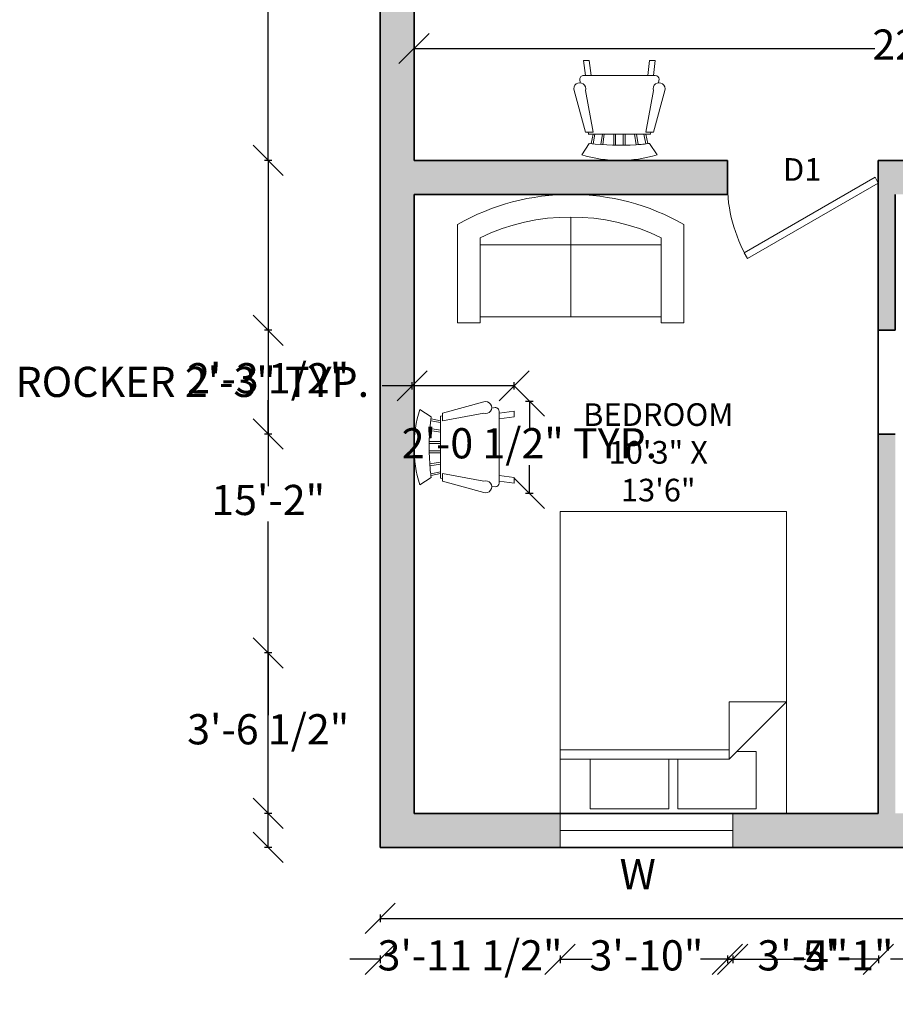
# Model space of a CAD drawing. Units: inches. Extents: x 2530 to 3100, y 543 to 1175.
# Tile 1 of 5: x 2530 to 2762, y 543 to 804. Entities that reach past the tile are written whole.
import ezdxf

# ---------------------------------------------------------------- set-up
doc = ezdxf.new("R2010")
doc.units = ezdxf.units.IN
for name, color, linetype, lineweight in [('A-ANNO-DIMS', 2, 'Continuous', 18), ('A-ANNO-TEXT', 7, 'Continuous', 18), ('A-AREA-IDEN', 7, 'Continuous', 18), ('A-DOOR', 3, 'Continuous', 18), ('A-FURN', 8, 'Continuous', 18), ('A-GLAZ', 4, 'Continuous', 18), ('A-WALL', 7, 'Continuous', 35), ('A-WALL-PATT', 30, 'Continuous', 13)]:
    doc.layers.add(name, color=color, linetype=linetype, lineweight=lineweight)
doc.styles.get("Standard").update_dxf_attribs({"font": 'arial.ttf'})
doc.dimstyles.new('ISO-25', dxfattribs={"dimtxt": 8, "dimasz": 8, "dimexe": 1, "dimexo": 1, "dimtad": 0, "dimtih": 1, "dimtoh": 1, "dimlunit": 3, "dimtxsty": 'Standard', "dimblk": 'OBLIQUE', "dimcen": 2.5, "dimadec": 0, "dimazin": 0, "dimtfac": 1, "dimtmove": 0, "dimatfit": 3, "dimfxl": 1, "dimfxlon": 1, "dimarcsym": 0})

# ---------------------------------------------------------------- blocks, each defined once
blk = doc.blocks.new('*U3')
for p, q in [((0, 0), (0, -6)), ((40, 0), (40, -6))]:
    blk.add_line(p, q)
blk.add_lwpolyline([(0, 0), (34.64, 20), (35.52, 18.48), (0.87, -1.52)], close=True)
blk.add_arc((0, 0), 40, 0, 30)
blk = doc.blocks.new('_Oblique')
at = {"color": 0, "linetype": 'ByBlock', "lineweight": -2}
blk.add_line((-0.5, -0.5), (0.5, 0.5), dxfattribs=at)
blk = doc.blocks.new('*D11')
at = {"layer": 'A-ANNO-DIMS', "color": 0, "lineweight": -2, "transparency": 16777216}
for p, q in [((2625.92, 566.6), (2625.92, 564.6)), ((3054.92, 566.6), (3054.92, 564.6)), ((2625.92, 565.6), (2826.05, 565.6)), ((3054.92, 565.6), (2854.78, 565.6))]:
    blk.add_line(p, q, dxfattribs=at)
at = {"layer": 'Defpoints', "color": 0, "transparency": 16777216}
for p in [(2625.92, 584.41), (3054.92, 584.41), (2625.92, 565.6)]:
    blk.add_point(p, dxfattribs=at)
at = {"layer": 'A-ANNO-DIMS', "color": 0, "lineweight": -2, "transparency": 16777216, "xscale": 8, "yscale": 8, "zscale": 8, "rotation": 180}
blk.add_blockref('_Oblique', (2625.92, 565.6), dxfattribs=at)
at = {"layer": 'A-ANNO-DIMS', "color": 0, "lineweight": -2, "transparency": 16777216, "xscale": 8, "yscale": 8, "zscale": 8}
blk.add_blockref('_Oblique', (3054.92, 565.6), dxfattribs=at)
at = {"layer": 'A-ANNO-DIMS', "color": 0, "transparency": 16777216, "insert": (2840.42, 565.6), "char_height": 8, "attachment_point": 5}
blk.add_mtext('35\'-9"', dxfattribs=at)
blk = doc.blocks.new('Chair - Rocking')
for p, q in [((-8, -4.5), (-10, -1.5)), ((8, -4.5), (10, -1.5)), ((-7.5, -4.5), (-7, -7)), ((-6.5, -7), (-7.02225, -4.43)), ((-4.5, -7), (-4.96674, -4.19951)), ((-4, -7), (-4.40532, -4.16272)), ((-1.5, -4.05012), (-1.5, -7)), ((-1, -7), (-1, -4.05012)), ((1, -7), (1, -4.04655)), ((1.5, -4.05012), (1.5, -7)), ((4, -7), (4.40187, -4.18694)), ((4.5, -7), (4.96761, -4.19437)), ((6.5, -7), (7, -4.4057)), ((7.5, -4.5), (7, -7)), ((-9, -7.5), (-12, -18.49999)), ((-7, -7.5), (-9, -7.5)), ((-9, -18.49999), (-7, -7.5)), ((-8.23428, -6.99939), (-8.3093, -7.47958)), ((-8.23041, -7), (8.23915, -7)), ((7, -7.5), (9, -7.5)), ((9, -18.49999), (7, -7.5)), ((8.31071, -7.48854), (8.23449, -7.00073)), ((9, -7.5), (12, -18.49999)), ((-10.36644, -20.64523), (-10.5, -21.49999)), ((10.5, -21.49999), (10.3575, -20.58798)), ((-9, -22.49999), (-9.5, -26.49999)), ((0, -22.49999), (-9.5, -22.49999)), ((-8, -26.49999), (-7.5, -22.49999)), ((0, -22.49999), (9.5, -22.49999)), ((8, -26.49999), (7.5, -22.49999)), ((9, -22.49999), (9.5, -26.49999)), ((-9.5, -26.49999), (-8, -26.49999)), ((9.5, -26.49999), (8, -26.49999))]:
    blk.add_line(p, q)
for centre, radius, start, end in [((0, -34.08333), 34.08333, 72.93847, 107.0615), ((0, -68.25004), 64.25, 93.92211, 97.15267), ((0, -68.25004), 64.25, 82.84733, 93.92211), ((-10.5, -18.99999), 1.58114, 161.5651, 18.43495), ((10.5, -18.99999), 1.58114, 161.5651, 18.43495), ((-9.5, -21.49999), 1, 180, 270), ((9.5, -21.49999), 1, 270, 0)]:
    blk.add_arc(centre, radius, start, end)
blk = doc.blocks.new('Bed - Queen')
for p, q in [((0, -80.00003), (0, 0)), ((0, 0), (59.99999, 0)), ((59.99999, 0), (59.99999, -80.00003)), ((7.99999, -1.2), (28.79998, -1.2)), ((7.99999, -14.4), (7.99999, -1.2)), ((28.79998, -1.2), (28.79998, -14.4)), ((31.19999, -1.2), (51.99999, -1.2)), ((31.19999, -14.4), (31.19999, -1.2)), ((51.99999, -1.2), (51.99999, -16.4)), ((0, -14.4), (44.8, -14.4)), ((59.99999, -29.6), (44.8, -14.4)), ((44.8, -14.4), (44.8, -29.6)), ((44.8, -16.8), (0, -16.8)), ((51.99999, -16.4), (46.79936, -16.4)), ((44.8, -29.6), (59.99999, -29.6)), ((59.99999, -80.00003), (0, -80.00003))]:
    blk.add_line(p, q)
blk = doc.blocks.new('Sofa - Roundback Loveseat 5 ft.')
for p, q in [((0, -32.44198), (0, -5.99998)), ((-24, -33.99998), (-24, -11.46958)), ((24.00004, -33.99998), (24.00004, -11.46958)), ((-23.9998, -13.38178), (23.99986, -13.38178)), ((-24, -32.44198), (24.00004, -32.44198))]:
    blk.add_line(p, q)
for points in [[(-24, -33.99998), (-30, -33.99998), (-30, -7.99998)], [(30.00004, -7.99998), (30.00004, -33.99998), (24.00004, -33.99998)]]:
    blk.add_lwpolyline(points)
for centre, radius, start, end in [((0, -60.24998), 60.24998, 60.13715, 119.8628), ((0, -61.38438), 55.38444, 64.32083, 115.6792)]:
    blk.add_arc(centre, radius, start, end)
blk = doc.blocks.new('*D26')
at = {"layer": 'A-ANNO-DIMS', "color": 0, "lineweight": -2, "transparency": 16777216}
for p, q in [((2634.42, 705.7), (2634.42, 707.7)), ((2661.42, 705.7), (2661.42, 707.7)), ((2634.42, 706.7), (2626.42, 706.7)), ((2661.42, 706.7), (2634.42, 706.7))]:
    blk.add_line(p, q, dxfattribs=at)
at = {"layer": 'Defpoints', "color": 0, "transparency": 16777216}
for p in [(2634.42, 706.7), (2634.42, 702.65), (2661.42, 702.65)]:
    blk.add_point(p, dxfattribs=at)
at = {"layer": 'A-ANNO-DIMS', "color": 0, "lineweight": -2, "transparency": 16777216, "xscale": 8, "yscale": 8, "zscale": 8, "rotation": 180}
blk.add_blockref('_Oblique', (2634.42, 706.7), dxfattribs=at)
at = {"layer": 'A-ANNO-DIMS', "color": 0, "lineweight": -2, "transparency": 16777216, "xscale": 8, "yscale": 8, "zscale": 8}
blk.add_blockref('_Oblique', (2661.42, 706.7), dxfattribs=at)
at = {"layer": 'A-ANNO-DIMS', "color": 0, "transparency": 16777216, "insert": (2576.16, 706.7), "char_height": 8, "attachment_point": 5}
blk.add_mtext('ROCKER 2\'-3" TYP.', dxfattribs=at)
blk = doc.blocks.new('*D27')
at = {"layer": 'A-ANNO-DIMS', "color": 0, "lineweight": -2, "transparency": 16777216}
for p, q in [((2664.47, 702.65), (2666.47, 702.65)), ((2665.47, 702.65), (2665.47, 695.19)), ((2665.47, 678.22), (2665.47, 685.67)), ((2664.47, 678.22), (2666.47, 678.22))]:
    blk.add_line(p, q, dxfattribs=at)
at = {"layer": 'Defpoints', "color": 0, "transparency": 16777216}
for p in [(2661.42, 702.65), (2665.47, 702.65), (2661.42, 678.22)]:
    blk.add_point(p, dxfattribs=at)
at = {"layer": 'A-ANNO-DIMS', "color": 0, "lineweight": -2, "transparency": 16777216, "xscale": 8, "yscale": 8, "zscale": 8}
for p, rotation in [((2665.47, 702.65), 90), ((2665.47, 678.22), 270)]:
    blk.add_blockref('_Oblique', p, dxfattribs=dict(at, rotation=rotation))
at = {"layer": 'A-ANNO-DIMS', "color": 0, "transparency": 16777216, "insert": (2665.47, 690.43), "char_height": 8, "attachment_point": 5}
blk.add_mtext('2\'-0 1/2" TYP.', dxfattribs=at)
blk = doc.blocks.new('*D46')
at = {"layer": 'A-ANNO-DIMS', "color": 0, "lineweight": -2, "transparency": 16777216}
for p, q in [((2634.92, 795.06), (2634.92, 797.06)), ((2634.92, 796.06), (2756.98, 796.06)), ((2907.92, 796.06), (2785.85, 796.06)), ((2907.92, 795.06), (2907.92, 797.06))]:
    blk.add_line(p, q, dxfattribs=at)
at = {"layer": 'Defpoints', "color": 0, "transparency": 16777216}
for p in [(2907.92, 796.06), (2634.92, 766.41), (2907.92, 766.41)]:
    blk.add_point(p, dxfattribs=at)
at = {"layer": 'A-ANNO-DIMS', "color": 0, "lineweight": -2, "transparency": 16777216, "xscale": 8, "yscale": 8, "zscale": 8, "rotation": 180}
blk.add_blockref('_Oblique', (2634.92, 796.06), dxfattribs=at)
at = {"layer": 'A-ANNO-DIMS', "color": 0, "lineweight": -2, "transparency": 16777216, "xscale": 8, "yscale": 8, "zscale": 8}
blk.add_blockref('_Oblique', (2907.92, 796.06), dxfattribs=at)
at = {"layer": 'A-ANNO-DIMS', "color": 0, "transparency": 16777216, "insert": (2771.42, 796.06), "char_height": 8, "attachment_point": 5}
blk.add_mtext('22\'-9"', dxfattribs=at)
blk = doc.blocks.new('*D47')
at = {"layer": 'A-ANNO-DIMS', "color": 0, "lineweight": -2, "transparency": 16777216}
for p, q in [((2597.27, 944.41), (2595.27, 944.41)), ((2596.27, 944.41), (2596.27, 860.12)), ((2596.27, 766.41), (2596.27, 850.7)), ((2597.27, 766.41), (2595.27, 766.41))]:
    blk.add_line(p, q, dxfattribs=at)
at = {"layer": 'Defpoints', "color": 0, "transparency": 16777216}
for p in [(2596.27, 944.41), (2634.92, 944.41), (2634.92, 766.41)]:
    blk.add_point(p, dxfattribs=at)
at = {"layer": 'A-ANNO-DIMS', "color": 0, "lineweight": -2, "transparency": 16777216, "xscale": 8, "yscale": 8, "zscale": 8}
for p, rotation in [((2596.27, 944.41), 90), ((2596.27, 766.41), 270)]:
    blk.add_blockref('_Oblique', p, dxfattribs=dict(at, rotation=rotation))
at = {"layer": 'A-ANNO-DIMS', "color": 0, "transparency": 16777216, "insert": (2596.27, 855.41), "char_height": 8, "attachment_point": 5}
blk.add_mtext('14\'-10"', dxfattribs=at)
blk = doc.blocks.new('*D48')
at = {"layer": 'A-ANNO-DIMS', "color": 0, "lineweight": -2, "transparency": 16777216}
for p, q in [((2597.27, 766.41), (2595.27, 766.41)), ((2596.27, 766.41), (2596.27, 680.12)), ((2596.27, 584.41), (2596.27, 670.7)), ((2597.27, 584.41), (2595.27, 584.41))]:
    blk.add_line(p, q, dxfattribs=at)
at = {"layer": 'Defpoints', "color": 0, "transparency": 16777216}
for p in [(2596.27, 766.41), (2634.92, 766.41), (2625.92, 584.41)]:
    blk.add_point(p, dxfattribs=at)
at = {"layer": 'A-ANNO-DIMS', "color": 0, "lineweight": -2, "transparency": 16777216, "xscale": 8, "yscale": 8, "zscale": 8}
for p, rotation in [((2596.27, 766.41), 90), ((2596.27, 584.41), 270)]:
    blk.add_blockref('_Oblique', p, dxfattribs=dict(at, rotation=rotation))
at = {"layer": 'A-ANNO-DIMS', "color": 0, "transparency": 16777216, "insert": (2596.27, 675.41), "char_height": 8, "attachment_point": 5}
blk.add_mtext('15\'-2"', dxfattribs=at)
blk = doc.blocks.new('*D56')
at = {"layer": 'A-ANNO-DIMS', "color": 0, "lineweight": -2, "transparency": 16777216}
for p, q in [((2625.92, 555.76), (2625.92, 553.76)), ((2673.58, 555.76), (2673.58, 553.76)), ((2625.92, 554.76), (2617.92, 554.76)), ((2625.92, 554.76), (2626.07, 554.76)), ((2673.58, 554.76), (2673.43, 554.76)), ((2673.58, 554.76), (2681.58, 554.76))]:
    blk.add_line(p, q, dxfattribs=at)
at = {"layer": 'Defpoints', "color": 0, "transparency": 16777216}
for p in [(2625.92, 584.41), (2673.58, 584.41), (2673.58, 554.76)]:
    blk.add_point(p, dxfattribs=at)
at = {"layer": 'A-ANNO-DIMS', "color": 0, "lineweight": -2, "transparency": 16777216, "xscale": 8, "yscale": 8, "zscale": 8}
blk.add_blockref('_Oblique', (2625.92, 554.76), dxfattribs=at)
at = {"layer": 'A-ANNO-DIMS', "color": 0, "lineweight": -2, "transparency": 16777216, "xscale": 8, "yscale": 8, "zscale": 8, "rotation": 180}
blk.add_blockref('_Oblique', (2673.58, 554.76), dxfattribs=at)
at = {"layer": 'A-ANNO-DIMS', "color": 0, "transparency": 16777216, "insert": (2649.75, 554.76), "char_height": 8, "attachment_point": 5}
blk.add_mtext('3\'-11 1/2"', dxfattribs=at)
blk = doc.blocks.new('*D57')
at = {"layer": 'A-ANNO-DIMS', "color": 0, "lineweight": -2, "transparency": 16777216}
for p, q in [((2673.58, 555.76), (2673.58, 553.76)), ((2719.35, 555.76), (2719.35, 553.76)), ((2673.58, 554.76), (2682.1, 554.76)), ((2719.35, 554.76), (2710.83, 554.76))]:
    blk.add_line(p, q, dxfattribs=at)
at = {"layer": 'Defpoints', "color": 0, "transparency": 16777216}
for p in [(2673.58, 584.41), (2719.35, 584.41), (2719.35, 554.76)]:
    blk.add_point(p, dxfattribs=at)
at = {"layer": 'A-ANNO-DIMS', "color": 0, "lineweight": -2, "transparency": 16777216, "xscale": 8, "yscale": 8, "zscale": 8, "rotation": 180}
blk.add_blockref('_Oblique', (2673.58, 554.76), dxfattribs=at)
at = {"layer": 'A-ANNO-DIMS', "color": 0, "lineweight": -2, "transparency": 16777216, "xscale": 8, "yscale": 8, "zscale": 8}
blk.add_blockref('_Oblique', (2719.35, 554.76), dxfattribs=at)
at = {"layer": 'A-ANNO-DIMS', "color": 0, "transparency": 16777216, "insert": (2696.47, 554.76), "char_height": 8, "attachment_point": 5}
blk.add_mtext('3\'-10"', dxfattribs=at)
blk = doc.blocks.new('*D58')
at = {"layer": 'A-ANNO-DIMS', "color": 0, "lineweight": -2, "transparency": 16777216}
for p, q in [((2719.35, 555.76), (2719.35, 553.76)), ((2780.42, 555.76), (2780.42, 553.76)), ((2719.35, 554.76), (2738.63, 554.76)), ((2780.42, 554.76), (2761.14, 554.76))]:
    blk.add_line(p, q, dxfattribs=at)
at = {"layer": 'Defpoints', "color": 0, "transparency": 16777216}
for p in [(2719.35, 584.41), (2780.42, 584.41), (2780.42, 554.76)]:
    blk.add_point(p, dxfattribs=at)
at = {"layer": 'A-ANNO-DIMS', "color": 0, "lineweight": -2, "transparency": 16777216, "xscale": 8, "yscale": 8, "zscale": 8, "rotation": 180}
blk.add_blockref('_Oblique', (2719.35, 554.76), dxfattribs=at)
at = {"layer": 'A-ANNO-DIMS', "color": 0, "lineweight": -2, "transparency": 16777216, "xscale": 8, "yscale": 8, "zscale": 8}
blk.add_blockref('_Oblique', (2780.42, 554.76), dxfattribs=at)
at = {"layer": 'A-ANNO-DIMS', "color": 0, "transparency": 16777216, "insert": (2749.88, 554.76), "char_height": 8, "attachment_point": 5}
blk.add_mtext('5\'-1"', dxfattribs=at)
blk = doc.blocks.new('*D64')
at = {"layer": 'A-ANNO-DIMS', "color": 0, "lineweight": -2, "transparency": 16777216}
for p, q in [((2717.92, 555.76), (2717.92, 553.76)), ((2757.92, 555.76), (2757.92, 553.76)), ((2717.92, 554.76), (2726.66, 554.76)), ((2757.92, 554.76), (2749.17, 554.76))]:
    blk.add_line(p, q, dxfattribs=at)
at = {"layer": 'Defpoints', "color": 0, "transparency": 16777216}
for p in [(2717.92, 757.41), (2757.92, 757.41), (2757.92, 554.76)]:
    blk.add_point(p, dxfattribs=at)
at = {"layer": 'A-ANNO-DIMS', "color": 0, "lineweight": -2, "transparency": 16777216, "xscale": 8, "yscale": 8, "zscale": 8, "rotation": 180}
blk.add_blockref('_Oblique', (2717.92, 554.76), dxfattribs=at)
at = {"layer": 'A-ANNO-DIMS', "color": 0, "lineweight": -2, "transparency": 16777216, "xscale": 8, "yscale": 8, "zscale": 8}
blk.add_blockref('_Oblique', (2757.92, 554.76), dxfattribs=at)
at = {"layer": 'A-ANNO-DIMS', "color": 0, "transparency": 16777216, "insert": (2737.92, 554.76), "char_height": 8, "attachment_point": 5}
blk.add_mtext('3\'-4"', dxfattribs=at)
blk = doc.blocks.new('*D68')
at = {"layer": 'A-ANNO-DIMS', "color": 0, "lineweight": -2, "transparency": 16777216}
for p, q in [((2597.27, 635.91), (2595.27, 635.91)), ((2596.27, 635.91), (2596.27, 619.42)), ((2596.27, 593.41), (2596.27, 609.89)), ((2597.27, 593.41), (2595.27, 593.41))]:
    blk.add_line(p, q, dxfattribs=at)
at = {"layer": 'Defpoints', "color": 0, "transparency": 16777216}
for p in [(2596.27, 635.91), (2927.92, 635.91), (2927.92, 593.41)]:
    blk.add_point(p, dxfattribs=at)
at = {"layer": 'A-ANNO-DIMS', "color": 0, "lineweight": -2, "transparency": 16777216, "xscale": 8, "yscale": 8, "zscale": 8}
for p, rotation in [((2596.27, 635.91), 90), ((2596.27, 593.41), 270)]:
    blk.add_blockref('_Oblique', p, dxfattribs=dict(at, rotation=rotation))
at = {"layer": 'A-ANNO-DIMS', "color": 0, "transparency": 16777216, "insert": (2596.27, 614.66), "char_height": 8, "attachment_point": 5}
blk.add_mtext('3\'-6 1/2"', dxfattribs=at)
blk = doc.blocks.new('*D83')
at = {"layer": 'A-ANNO-DIMS', "color": 0, "lineweight": -2, "transparency": 16777216}
for p, q in [((2597.27, 721.41), (2595.27, 721.41)), ((2596.27, 721.41), (2596.27, 712.42)), ((2596.27, 693.91), (2596.27, 702.89)), ((2597.27, 693.91), (2595.27, 693.91))]:
    blk.add_line(p, q, dxfattribs=at)
at = {"layer": 'Defpoints', "color": 0, "transparency": 16777216}
for p in [(2596.27, 721.41), (2757.92, 721.41), (2757.92, 693.91)]:
    blk.add_point(p, dxfattribs=at)
at = {"layer": 'A-ANNO-DIMS', "color": 0, "lineweight": -2, "transparency": 16777216, "xscale": 8, "yscale": 8, "zscale": 8}
for p, rotation in [((2596.27, 721.41), 90), ((2596.27, 693.91), 270)]:
    blk.add_blockref('_Oblique', p, dxfattribs=dict(at, rotation=rotation))
at = {"layer": 'A-ANNO-DIMS', "color": 0, "transparency": 16777216, "insert": (2596.27, 707.66), "char_height": 8, "attachment_point": 5}
blk.add_mtext('2\'-3 1/2"', dxfattribs=at)

msp = doc.modelspace()

# ---------------------------------------------------------------- hatches: boundary and pattern name
at = {"layer": 'A-WALL-PATT'}
h = msp.add_hatch(color=256, dxfattribs=at)
h.dxf.hatch_style = 1
h.paths.add_polyline_path([(2676.945, 1133.407), (2625.918, 1133.407), (2625.918, 584.407), (2673.585, 584.407), (2673.585, 593.407), (2634.918, 593.407), (2634.918, 757.407), (2717.918, 757.407), (2717.918, 766.407), (2634.918, 766.407), (2634.918, 944.407), (2772.918, 944.407), (2772.918, 948.407), (2634.918, 948.407), (2634.918, 1124.407), (2676.945, 1124.407)])
h.paths.add_polyline_path([(2822.346, 1133.407), (2739.946, 1133.407), (2739.946, 1124.407), (2808.918, 1124.407), (2808.918, 1070.407), (2812.918, 1070.407), (2812.918, 1124.407), (2822.346, 1124.407)])
h.paths.add_polyline_path([(2939.91, 1133.407), (2855.561, 1133.407), (2855.561, 1124.407), (2867.918, 1124.407), (2867.918, 1038.407), (2808.918, 1038.407), (2808.918, 944.407), (2871.918, 944.407), (2871.918, 1002.407), (2867.918, 1002.407), (2867.918, 948.407), (2812.918, 948.407), (2812.918, 1034.407), (2871.918, 1034.407), (2871.918, 1124.407), (2939.91, 1124.407)])
h.paths.add_polyline_path([(3054.918, 1133.407), (2997.969, 1133.407), (2997.969, 1124.407), (3045.918, 1124.407), (3045.918, 948.407), (2907.918, 948.407), (2907.918, 928.407), (2911.918, 928.407), (2911.918, 944.407), (2952.418, 944.407), (2952.418, 872.407), (2911.918, 872.407), (2911.918, 888.407), (2907.918, 888.407), (2907.918, 861.407), (2911.918, 861.407), (2911.918, 867.407), (2956.918, 867.407), (2956.918, 944.407), (3045.918, 944.407), (3045.918, 872.407), (2988.918, 872.407), (2988.918, 867.407), (3045.918, 867.407), (3045.918, 766.407), (2986.918, 766.407), (2986.918, 757.407), (3045.918, 757.407), (3045.918, 593.407), (2906.263, 593.407), (2906.263, 584.407), (3054.918, 584.407)])
h.paths.add_polyline_path([(2780.418, 593.407), (2762.418, 593.407), (2762.418, 693.907), (2757.918, 693.907), (2757.918, 593.407), (2719.35, 593.407), (2719.35, 584.407), (2780.418, 584.407)])
h.paths.add_polyline_path([(2846.356, 593.407), (2826.918, 593.407), (2826.918, 757.407), (2826.918, 766.407), (2822.418, 766.407), (2822.418, 693.907), (2794.418, 693.907), (2794.418, 689.407), (2822.418, 689.407), (2822.418, 593.407), (2804.418, 593.407), (2804.418, 584.407), (2846.356, 584.407)])
h.paths.add_polyline_path([(2938.918, 766.407), (2911.918, 766.407), (2911.918, 829.407), (2907.918, 829.407), (2907.918, 766.407), (2886.918, 766.407), (2886.918, 757.407), (2938.918, 757.407)])
h.paths.add_polyline_path([(2822.418, 766.407), (2757.918, 766.407), (2757.918, 757.407), (2757.918, 721.407), (2762.418, 721.407), (2762.418, 757.407), (2822.418, 757.407)])

# ---------------------------------------------------------------- linework, layer by layer
at = {"layer": 'A-GLAZ'}
for p, q in [((2673.585, 593.407), (2673.585, 584.407)), ((2719.35, 593.407), (2719.35, 584.407)), ((2673.585, 588.907), (2719.35, 588.907))]:
    msp.add_line(p, q, dxfattribs=at)
at = {"layer": 'A-WALL'}
for p, q in [((2625.918, 1133.407), (2625.918, 584.407)), ((2634.918, 944.407), (2634.918, 766.407)), ((2717.918, 766.407), (2634.918, 766.407)), ((2717.918, 757.407), (2717.918, 766.407)), ((2757.918, 757.407), (2757.918, 766.407)), ((2826.918, 766.407), (2757.918, 766.407)), ((2634.918, 757.407), (2634.918, 593.407)), ((2717.918, 757.407), (2634.918, 757.407)), ((2757.918, 757.407), (2757.918, 593.407)), ((2762.418, 757.407), (2762.418, 721.407)), ((2762.418, 721.407), (2757.918, 721.407)), ((2757.918, 693.907), (2762.418, 693.907)), ((2634.918, 593.407), (2757.918, 593.407)), ((2625.918, 584.407), (3054.918, 584.407))]:
    msp.add_line(p, q, dxfattribs=at)

# ---------------------------------------------------------------- block references
at = {"layer": 'A-DOOR', "rotation": 180}
msp.add_blockref('*U3', (2757.918, 760.407), dxfattribs=at)
at = {"layer": 'A-FURN'}
for p, rotation in [((2689.322, 766.407), 180), ((2634.918, 690.433), 89.99999999999999)]:
    msp.add_blockref('Chair - Rocking', p, dxfattribs=dict(at, rotation=rotation))
msp.add_blockref('Sofa - Roundback Loveseat 5 ft.', (2676.418, 757.407), dxfattribs=at)
at = {"layer": 'A-FURN', "xscale": -1, "rotation": 180}
msp.add_blockref('Bed - Queen', (2673.585, 593.407), dxfattribs=at)

# ---------------------------------------------------------------- texts
at = {"layer": 'A-ANNO-TEXT', "attachment_point": 1}
for s, insert, char_height in [('\\pxqc;D1', (2728.512, 767.005), 6), ('\\pxqc;W', (2684.927, 581.318), 8)]:
    msp.add_mtext_dynamic_manual_height_columns(s, width=18.48176, gutter_width=12.5, heights=[0], dxfattribs=dict(at, insert=insert, char_height=char_height))
at = {"layer": 'A-AREA-IDEN', "insert": (2675.776, 702.062), "char_height": 6, "attachment_point": 1}
msp.add_mtext_dynamic_manual_height_columns('\\pxqc;BEDROOM\\P10\'3" X 13\'6"', width=47.65744, gutter_width=12.5, heights=[0], dxfattribs=at)

# ---------------------------------------------------------------- dimensions: what is measured, and where the dimension line sits
at = {"layer": 'A-ANNO-DIMS'}
for base, p1, p2, picture, middle in [((2596.268, 944.407), (2634.918, 766.407), (2634.918, 944.407), '*D47', (2596.268, 855.407)), ((2596.268, 766.407), (2625.918, 584.407), (2634.918, 766.407), '*D48', (2596.268, 675.407)), ((2596.268, 721.407), (2757.918, 693.907), (2757.918, 721.407), '*D83', (2596.268, 707.657)), ((2596.268, 635.907), (2927.918, 593.407), (2927.918, 635.907), '*D68', (2596.268, 614.657))]:
    dim = msp.add_linear_dim(base=base, p1=p1, p2=p2, angle=90, dimstyle='ISO-25', override={"dimdec": 1, "dimlfac": 1, "dimrnd": 0, "dimzin": 1, "dimdsep": 46, "dimlunit": 4, "dimfrac": 2}, dxfattribs=at)
    dim.commit()
    dim.dimension.update_dxf_attribs({"geometry": picture, "text_midpoint": middle})
for base, p1, p2, override, picture, middle in [((2907.918, 796.057), (2634.918, 766.407), (2907.918, 766.407), {"dimdec": 1, "dimlfac": 1, "dimrnd": 0, "dimzin": 1, "dimdsep": 46, "dimlunit": 4, "dimfrac": 2}, '*D46', (2771.418, 796.057)), ((2757.918, 554.757), (2717.918, 757.407), (2757.918, 757.407), {"dimdec": 1, "dimlfac": 1, "dimrnd": 0, "dimzin": 1, "dimdsep": 46, "dimlunit": 4, "dimfrac": 2}, '*D64', (2737.918, 554.757)), ((2673.585, 554.757), (2625.918, 584.407), (2673.585, 584.407), {"dimdec": 1, "dimlfac": 1, "dimrnd": 0, "dimzin": 1, "dimdsep": 46, "dimlunit": 4, "dimfrac": 2}, '*D56', (2649.751, 554.757)), ((2625.918, 565.597), (3054.918, 584.407), (2625.918, 584.407), {"dimclrd": 0, "dimclre": 0, "dimclrt": 0}, '*D11', (2840.418, 565.597)), ((2719.35, 554.757), (2673.585, 584.407), (2719.35, 584.407), {"dimdec": 1, "dimlfac": 1, "dimrnd": 0, "dimzin": 1, "dimdsep": 46, "dimlunit": 4, "dimfrac": 2}, '*D57', (2696.468, 554.757)), ((2780.418, 554.757), (2719.35, 584.407), (2780.418, 584.407), {"dimdec": 1, "dimlfac": 1, "dimrnd": 0, "dimzin": 1, "dimdsep": 46, "dimlunit": 4, "dimfrac": 2}, '*D58', (2749.884, 554.757))]:
    dim = msp.add_linear_dim(base=base, p1=p1, p2=p2, dimstyle='ISO-25', override=override, dxfattribs=at)
    dim.commit()
    dim.dimension.update_dxf_attribs({"geometry": picture, "text_midpoint": middle})
for base, p1, p2, angle, text, picture, middle in [((2634.418, 706.701), (2661.418, 702.651), (2634.418, 702.651), 180, 'ROCKER <> TYP.', '*D26', (2576.158, 706.701)), ((2665.468, 702.651), (2661.418, 678.216), (2661.418, 702.651), 90, '<> TYP.', '*D27', (2665.468, 690.433))]:
    dim = msp.add_linear_dim(base=base, p1=p1, p2=p2, angle=angle, text=text, dimstyle='ISO-25', override={"dimdec": 1, "dimlfac": 1, "dimrnd": 0, "dimzin": 1, "dimdsep": 46, "dimlunit": 4, "dimfrac": 2}, dxfattribs=at)
    dim.commit()
    dim.dimension.update_dxf_attribs({"geometry": picture, "text_midpoint": middle})

doc.saveas('drawing.dxf')
